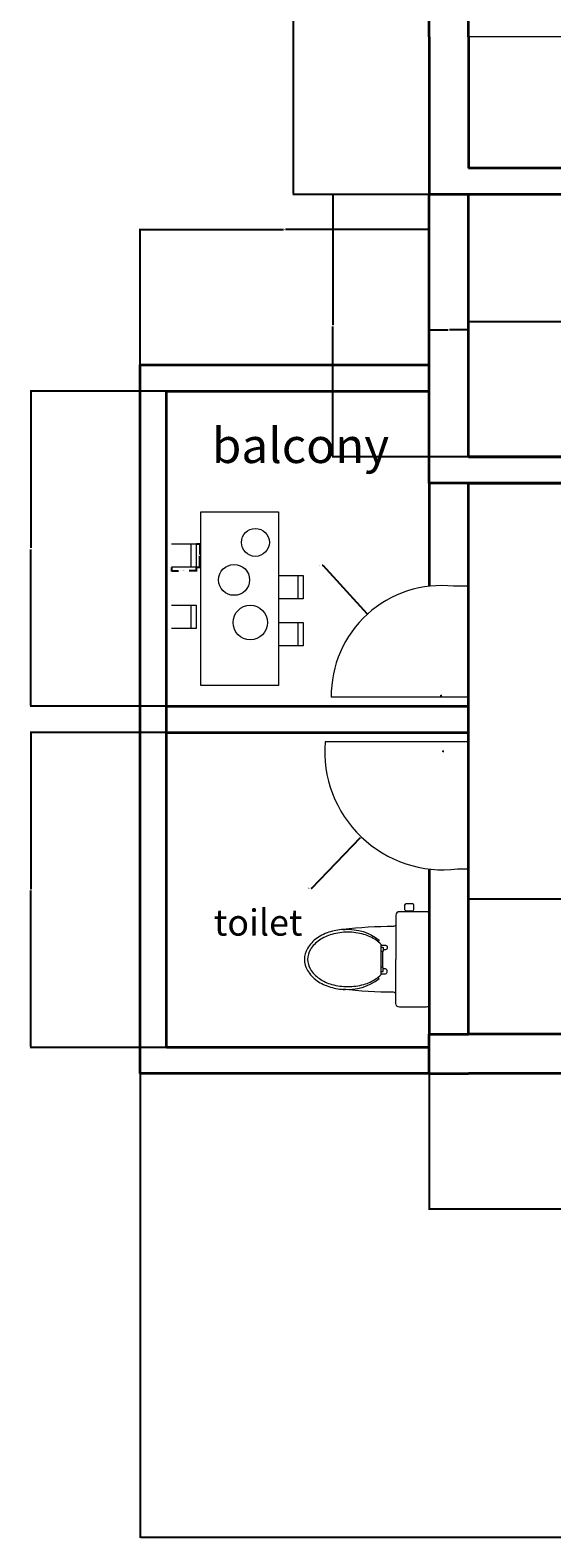
# Model space of a CAD drawing. Units: inches. Extents: x 177 to 785, y -381 to 206.
# Tile 1 of 5: x 177 to 296, y -381 to -37. Entities that reach past the tile are written whole.
import ezdxf

# ---------------------------------------------------------------- set-up
doc = ezdxf.new("R2010")
doc.units = ezdxf.units.IN
doc.header["$MEASUREMENT"] = 0
for name, color, linetype, lineweight in [('A-ANNO-DIMS', 2, 'Continuous', 18), ('A-AREA-IDEN', 7, 'Continuous', 20), ('A-DOOR', 4, 'Continuous', 18), ('A-FLOR-FIXT', 8, 'Continuous', 18), ('A-FURN', 2, 'Continuous', 18), ('A-WALL', 7, 'Continuous', 35), ('WC-Detail_dwgmodels.com', 9, 'Continuous', 13), ('WC-Outline_dwgmodels.com', 8, 'Continuous', 18)]:
    doc.layers.add(name, color=color, linetype=linetype, lineweight=lineweight)
doc.styles.get("Standard").update_dxf_attribs({"font": 'arial.ttf'})
doc.dimstyles.get("Standard").update_dxf_attribs({"dimtxt": 0.18, "dimasz": 0.18, "dimexe": 0.18, "dimexo": 0.0625, "dimgap": 0.09, "dimtad": 0, "dimtih": 1, "dimtoh": 1, "dimdec": 4, "dimzin": 0, "dimdsep": 46, "dimtxsty": 'Standard', "dimcen": 0.09, "dimadec": 0, "dimazin": 0, "dimtfac": 1, "dimtdec": 4, "dimtofl": 0, "dimtmove": 0, "dimatfit": 3, "dimfxl": 1, "dimtolj": 1, "dimtzin": 0, "dimarcsym": 0})

# ---------------------------------------------------------------- blocks, each defined once
blk = doc.blocks.new('BED-DOUBLE')
blk.add_line((58.96, 86.04), (58.96, 0))
for points in [[(0, 86.04), (102.05, 86.04), (102.05, 0), (0, 0)], [(70.1, 73.56), (83.84, 73.56), (83.84, 43.2), (70.1, 43.2)], [(70.1, 37.79), (83.84, 37.79), (83.84, 7.42), (70.1, 7.42)]]:
    blk.add_lwpolyline(points, close=True)
blk = doc.blocks.new('CHAIR-BALCONY-SMALL')
for p, q in [((0, 5.34), (4.46, 5.34)), ((4.46, 5.34), (4.46, 0)), ((4.46, 5.34), (5.66, 5.34)), ((5.66, 5.34), (5.66, 0)), ((4.46, 0), (0, 0)), ((5.66, 0), (4.46, 0))]:
    blk.add_line(p, q)
blk = doc.blocks.new('WC-PAN-AND-SEAT')
for points in [[(0, 20.91, -0.279901), (0.43, 20.4, 0.030761), (1.12, 8.8, 16.522544)], [(15.88, 20.91, 0.279901), (15.45, 20.4, -0.030761), (14.76, 8.8, -16.522544)], [(1.72, 9.92, 0.068564), (2.22, 6.28, 0.080689), (3.54, 3.43, 0.107047), (5.7, 1.38, 0.137952), (7.94, 0.75, 0.137952), (10.18, 1.38, 0.107047), (12.34, 3.43, 0.080689), (13.66, 6.28, 0.068564), (14.16, 9.92, 0.068564), (13.66, 13.57, 0.080689), (12.34, 16.41, 0.049741), (11.45, 17.48, 0.137952)], [(4.44, 17.48, 0.049741), (3.54, 16.41, 0.080689), (2.22, 13.57, 0.068564), (1.72, 9.92, 0.068564)], [(1.08, 9.29, -0.186192), (3.55, 17.08), (3.86, 16.84)], [(14.76, 8.8, 0.197511), (12.33, 17.08), (12.02, 16.84)], [(1.07, 9.29, 0.059006), (1.61, 5.99, 0.081908), (3.07, 2.91, 0.106902), (5.45, 0.69, 0.135271), (7.94, 0, 0.135271)], [(1.12, 8.8, -0.010918), (1.08, 9.29)], [(7.94, 0, 0.135271), (10.44, 0.69, 0.106902), (12.81, 2.91, 0.081908), (14.28, 5.99, 0.059006), (14.82, 9.29, 0.070136)]]:
    blk.add_lwpolyline(points, format="xyb")
blk.add_lwpolyline([(4.44, 17.48), (11.45, 17.48)])
blk = doc.blocks.new('*D11')
at = {"layer": 'A-ANNO-DIMS', "color": 0, "lineweight": -2, "transparency": 16777216}
for p, q in [((209.45, -159.41), (209.45, -160.37)), ((209.63, -160.19), (211.07, -160.19)), ((214.93, -160.19), (213.49, -160.19)), ((215.11, -159.41), (215.11, -160.37))]:
    blk.add_line(p, q, dxfattribs=at)
at = {"layer": 'A-ANNO-DIMS', "color": 0, "transparency": 16777216}
for points in [[(209.63, -160.16), (209.63, -160.22), (209.45, -160.19)], [(214.93, -160.16), (214.93, -160.22), (215.11, -160.19)]]:
    blk.add_solid(points, dxfattribs=at)
at = {"layer": 'Defpoints', "color": 0, "transparency": 16777216}
for p in [(209.45, -159.35), (215.11, -159.35), (215.11, -160.19)]:
    blk.add_point(p, dxfattribs=at)
at = {"layer": 'A-ANNO-DIMS', "color": 0, "transparency": 16777216, "insert": (212.28, -160.19), "char_height": 0.18, "attachment_point": 5}
blk.add_mtext('\\A1;SIDE CHAIR 6 TYP.', dxfattribs=at)
blk = doc.blocks.new('*D12')
at = {"layer": 'A-ANNO-DIMS', "color": 0, "lineweight": -2, "transparency": 16777216}
for p, q in [((215.18, -154.01), (216.14, -154.01)), ((215.96, -154.19), (215.96, -156.5)), ((215.96, -159.17), (215.96, -156.86)), ((215.18, -159.35), (216.14, -159.35))]:
    blk.add_line(p, q, dxfattribs=at)
at = {"layer": 'A-ANNO-DIMS', "color": 0, "transparency": 16777216}
for points in [[(215.93, -154.19), (215.99, -154.19), (215.96, -154.01)], [(215.93, -159.17), (215.99, -159.17), (215.96, -159.35)]]:
    blk.add_solid(points, dxfattribs=at)
at = {"layer": 'Defpoints', "color": 0, "transparency": 16777216}
for p in [(215.11, -154.01), (215.96, -154.01), (215.11, -159.35)]:
    blk.add_point(p, dxfattribs=at)
at = {"layer": 'A-ANNO-DIMS', "color": 0, "transparency": 16777216, "insert": (215.96, -156.68), "char_height": 0.18, "attachment_point": 5}
blk.add_mtext('\\A1;5 TYP.', dxfattribs=at)
blk = doc.blocks.new('*D23')
at = {"layer": 'A-ANNO-DIMS', "color": 0, "lineweight": -2, "transparency": 16777216}
for p, q in [((754.33, -257.2), (754.33, -381.27)), ((202.33, -275.2), (202.33, -381.27)), ((202.51, -381.09), (478.04, -381.09)), ((754.15, -381.09), (478.62, -381.09))]:
    blk.add_line(p, q, dxfattribs=at)
at = {"layer": 'A-ANNO-DIMS', "color": 0, "transparency": 16777216}
for points in [[(202.51, -381.06), (202.51, -381.12), (202.33, -381.09)], [(754.15, -381.06), (754.15, -381.12), (754.33, -381.09)]]:
    blk.add_solid(points, dxfattribs=at)
at = {"layer": 'Defpoints', "color": 0, "transparency": 16777216}
for p in [(754.33, -257.14), (202.33, -275.14), (754.33, -381.09)]:
    blk.add_point(p, dxfattribs=at)
at = {"layer": 'A-ANNO-DIMS', "color": 0, "transparency": 16777216, "insert": (478.33, -381.09), "char_height": 0.18, "attachment_point": 5}
blk.add_mtext('\\A1;552', dxfattribs=at)
blk = doc.blocks.new('*D25')
at = {"layer": 'A-ANNO-DIMS', "color": 0, "lineweight": -2, "transparency": 16777216}
for p, q in [((202.33, -113.08), (202.33, -82.01)), ((202.51, -82.19), (235.11, -82.19)), ((268.15, -82.19), (235.55, -82.19)), ((268.33, -113.08), (268.33, -82.01))]:
    blk.add_line(p, q, dxfattribs=at)
at = {"layer": 'A-ANNO-DIMS', "color": 0, "transparency": 16777216}
for points in [[(202.51, -82.16), (202.51, -82.22), (202.33, -82.19)], [(268.15, -82.16), (268.15, -82.22), (268.33, -82.19)]]:
    blk.add_solid(points, dxfattribs=at)
at = {"layer": 'Defpoints', "color": 0, "transparency": 16777216}
for p in [(268.33, -82.19), (202.33, -113.14), (268.33, -113.14)]:
    blk.add_point(p, dxfattribs=at)
at = {"layer": 'A-ANNO-DIMS', "color": 0, "transparency": 16777216, "insert": (235.33, -82.19), "char_height": 0.18, "attachment_point": 5}
blk.add_mtext('\\A1;66', dxfattribs=at)
blk = doc.blocks.new('*D37')
at = {"layer": 'A-ANNO-DIMS', "color": 0, "lineweight": -2, "transparency": 16777216}
for p, q in [((268.27, 102.86), (237.2, 102.86)), ((237.38, 102.68), (237.38, 14.54)), ((237.38, -73.96), (237.38, 14.18)), ((268.27, -74.14), (237.2, -74.14))]:
    blk.add_line(p, q, dxfattribs=at)
at = {"layer": 'A-ANNO-DIMS', "color": 0, "transparency": 16777216}
for points in [[(237.35, 102.68), (237.41, 102.68), (237.38, 102.86)], [(237.35, -73.96), (237.41, -73.96), (237.38, -74.14)]]:
    blk.add_solid(points, dxfattribs=at)
at = {"layer": 'Defpoints', "color": 0, "transparency": 16777216}
for p in [(237.38, 102.86), (268.33, 102.86), (268.33, -74.14)]:
    blk.add_point(p, dxfattribs=at)
at = {"layer": 'A-ANNO-DIMS', "color": 0, "transparency": 16777216, "insert": (237.38, 14.36), "char_height": 0.18, "attachment_point": 5}
blk.add_mtext('\\A1;177', dxfattribs=at)
blk = doc.blocks.new('*D41')
at = {"layer": 'A-ANNO-DIMS', "color": 0, "lineweight": -2, "transparency": 16777216}
for p, q in [((277.33, -134.08), (277.33, -103.01)), ((277.51, -103.19), (321.11, -103.19)), ((365.15, -103.19), (321.55, -103.19)), ((365.33, -134.08), (365.33, -103.01))]:
    blk.add_line(p, q, dxfattribs=at)
at = {"layer": 'A-ANNO-DIMS', "color": 0, "transparency": 16777216}
for points in [[(277.51, -103.16), (277.51, -103.22), (277.33, -103.19)], [(365.15, -103.16), (365.15, -103.22), (365.33, -103.19)]]:
    blk.add_solid(points, dxfattribs=at)
at = {"layer": 'Defpoints', "color": 0, "transparency": 16777216}
for p in [(365.33, -103.19), (277.33, -134.14), (365.33, -134.14)]:
    blk.add_point(p, dxfattribs=at)
at = {"layer": 'A-ANNO-DIMS', "color": 0, "transparency": 16777216, "insert": (321.33, -103.19), "char_height": 0.18, "attachment_point": 5}
blk.add_mtext('\\A1;88', dxfattribs=at)
blk = doc.blocks.new('*D42')
at = {"layer": 'A-ANNO-DIMS', "color": 0, "lineweight": -2, "transparency": 16777216}
for p, q in [((277.27, -74.14), (246.2, -74.14)), ((246.38, -74.32), (246.38, -103.96)), ((246.38, -133.96), (246.38, -104.32)), ((277.27, -134.14), (246.2, -134.14))]:
    blk.add_line(p, q, dxfattribs=at)
at = {"layer": 'A-ANNO-DIMS', "color": 0, "transparency": 16777216}
for points in [[(246.35, -74.32), (246.41, -74.32), (246.38, -74.14)], [(246.35, -133.96), (246.41, -133.96), (246.38, -134.14)]]:
    blk.add_solid(points, dxfattribs=at)
at = {"layer": 'Defpoints', "color": 0, "transparency": 16777216}
for p in [(246.38, -74.14), (277.33, -74.14), (277.33, -134.14)]:
    blk.add_point(p, dxfattribs=at)
at = {"layer": 'A-ANNO-DIMS', "color": 0, "transparency": 16777216, "insert": (246.38, -104.14), "char_height": 0.18, "attachment_point": 5}
blk.add_mtext('\\A1;60', dxfattribs=at)
blk = doc.blocks.new('*D43')
at = {"layer": 'A-ANNO-DIMS', "color": 0, "lineweight": -2, "transparency": 16777216}
for p, q in [((208.27, -119.14), (177.2, -119.14)), ((177.38, -119.32), (177.38, -154.96)), ((177.38, -190.96), (177.38, -155.32)), ((208.27, -191.14), (177.2, -191.14))]:
    blk.add_line(p, q, dxfattribs=at)
at = {"layer": 'A-ANNO-DIMS', "color": 0, "transparency": 16777216}
for points in [[(177.35, -119.32), (177.41, -119.32), (177.38, -119.14)], [(177.35, -190.96), (177.41, -190.96), (177.38, -191.14)]]:
    blk.add_solid(points, dxfattribs=at)
at = {"layer": 'Defpoints', "color": 0, "transparency": 16777216}
for p in [(177.38, -119.14), (208.33, -119.14), (208.33, -191.14)]:
    blk.add_point(p, dxfattribs=at)
at = {"layer": 'A-ANNO-DIMS', "color": 0, "transparency": 16777216, "insert": (177.38, -155.14), "char_height": 0.18, "attachment_point": 5}
blk.add_mtext('\\A1;72', dxfattribs=at)
blk = doc.blocks.new('*D44')
at = {"layer": 'A-ANNO-DIMS', "color": 0, "lineweight": -2, "transparency": 16777216}
for p, q in [((208.27, -197.14), (177.2, -197.14)), ((177.38, -197.32), (177.38, -232.96)), ((177.38, -268.96), (177.38, -233.32)), ((208.27, -269.14), (177.2, -269.14))]:
    blk.add_line(p, q, dxfattribs=at)
at = {"layer": 'A-ANNO-DIMS', "color": 0, "transparency": 16777216}
for points in [[(177.35, -197.32), (177.41, -197.32), (177.38, -197.14)], [(177.35, -268.96), (177.41, -268.96), (177.38, -269.14)]]:
    blk.add_solid(points, dxfattribs=at)
at = {"layer": 'Defpoints', "color": 0, "transparency": 16777216}
for p in [(177.38, -197.14), (208.33, -197.14), (208.33, -269.14)]:
    blk.add_point(p, dxfattribs=at)
at = {"layer": 'A-ANNO-DIMS', "color": 0, "transparency": 16777216, "insert": (177.38, -233.14), "char_height": 0.18, "attachment_point": 5}
blk.add_mtext('\\A1;72', dxfattribs=at)
blk = doc.blocks.new('*D45')
at = {"layer": 'A-ANNO-DIMS', "color": 0, "lineweight": -2, "transparency": 16777216}
for p, q in [((277.33, -266.08), (277.33, -235.01)), ((277.51, -235.19), (370.05, -235.19)), ((463.15, -235.19), (370.61, -235.19)), ((463.33, -266.08), (463.33, -235.01))]:
    blk.add_line(p, q, dxfattribs=at)
at = {"layer": 'A-ANNO-DIMS', "color": 0, "transparency": 16777216}
for points in [[(277.51, -235.16), (277.51, -235.22), (277.33, -235.19)], [(463.15, -235.16), (463.15, -235.22), (463.33, -235.19)]]:
    blk.add_solid(points, dxfattribs=at)
at = {"layer": 'Defpoints', "color": 0, "transparency": 16777216}
for p in [(463.33, -235.19), (277.33, -266.14), (463.33, -266.14)]:
    blk.add_point(p, dxfattribs=at)
at = {"layer": 'A-ANNO-DIMS', "color": 0, "transparency": 16777216, "insert": (370.33, -235.19), "char_height": 0.18, "attachment_point": 5}
blk.add_mtext('\\A1;186', dxfattribs=at)
blk = doc.blocks.new('*D63')
at = {"layer": 'A-ANNO-DIMS', "color": 0, "lineweight": -2, "transparency": 16777216}
for p, q in [((268.33, -74.2), (268.33, -105.27)), ((277.33, -74.2), (277.33, -105.27)), ((268.51, -105.09), (272.68, -105.09)), ((277.15, -105.09), (272.98, -105.09))]:
    blk.add_line(p, q, dxfattribs=at)
at = {"layer": 'A-ANNO-DIMS', "color": 0, "transparency": 16777216}
for points in [[(268.51, -105.06), (268.51, -105.12), (268.33, -105.09)], [(277.15, -105.06), (277.15, -105.12), (277.33, -105.09)]]:
    blk.add_solid(points, dxfattribs=at)
at = {"layer": 'Defpoints', "color": 0, "transparency": 16777216}
for p in [(268.33, -74.14), (277.33, -74.14), (268.33, -105.09)]:
    blk.add_point(p, dxfattribs=at)
at = {"layer": 'A-ANNO-DIMS', "color": 0, "transparency": 16777216, "insert": (272.83, -105.09), "char_height": 0.18, "attachment_point": 5}
blk.add_mtext('\\A1;9', dxfattribs=at)
blk = doc.blocks.new('*D65')
at = {"layer": 'A-ANNO-DIMS', "color": 0, "lineweight": -2, "transparency": 16777216}
for p, q in [((268.33, -275.2), (268.33, -306.27)), ((362.7, -275.2), (362.7, -306.27)), ((268.51, -306.09), (315.12, -306.09)), ((362.52, -306.09), (315.91, -306.09))]:
    blk.add_line(p, q, dxfattribs=at)
at = {"layer": 'A-ANNO-DIMS', "color": 0, "transparency": 16777216}
for points in [[(268.51, -306.06), (268.51, -306.12), (268.33, -306.09)], [(362.52, -306.06), (362.52, -306.12), (362.7, -306.09)]]:
    blk.add_solid(points, dxfattribs=at)
at = {"layer": 'Defpoints', "color": 0, "transparency": 16777216}
for p in [(268.33, -275.14), (362.7, -275.14), (268.33, -306.09)]:
    blk.add_point(p, dxfattribs=at)
at = {"layer": 'A-ANNO-DIMS', "color": 0, "transparency": 16777216, "insert": (315.51, -306.09), "char_height": 0.18, "attachment_point": 5}
blk.add_mtext('\\A1;94.37', dxfattribs=at)
blk = doc.blocks.new('*D81')
at = {"layer": 'A-ANNO-DIMS', "color": 0, "lineweight": -2, "transparency": 16777216}
for p, q in [((271.49, -201.46), (271.67, -201.46)), ((271.58, -201.55), (271.58, -201.37)), ((241.55, -232.74), (252.69, -221.14)), ((241.37, -232.74), (241.55, -232.74))]:
    blk.add_line(p, q, dxfattribs=at)
at = {"layer": 'A-ANNO-DIMS', "color": 0, "transparency": 16777216}
blk.add_solid([(252.67, -221.12), (252.71, -221.16), (252.81, -221.01)], dxfattribs=at)
at = {"layer": 'Defpoints', "color": 0, "transparency": 16777216}
for p in [(271.58, -201.46), (252.81, -221.01)]:
    blk.add_point(p, dxfattribs=at)
at = {"layer": 'A-ANNO-DIMS', "color": 0, "transparency": 16777216, "insert": (240.98, -232.74), "char_height": 0.18, "attachment_point": 5}
blk.add_mtext('\\A1;R27.1', dxfattribs=at)
blk = doc.blocks.new('*D82')
at = {"layer": 'A-ANNO-DIMS', "color": 0, "lineweight": -2, "transparency": 16777216}
for p, q in [((243.91, -158.94), (244.09, -158.94)), ((244.09, -158.94), (254.11, -169.98)), ((271.04, -188.74), (271.22, -188.74)), ((271.13, -188.83), (271.13, -188.65))]:
    blk.add_line(p, q, dxfattribs=at)
at = {"layer": 'A-ANNO-DIMS', "color": 0, "transparency": 16777216}
blk.add_solid([(254.13, -169.96), (254.09, -170), (254.23, -170.12)], dxfattribs=at)
at = {"layer": 'Defpoints', "color": 0, "transparency": 16777216}
for p in [(254.23, -170.12), (271.13, -188.74)]:
    blk.add_point(p, dxfattribs=at)
at = {"layer": 'A-ANNO-DIMS', "color": 0, "transparency": 16777216, "insert": (243.36, -158.94), "char_height": 0.18, "attachment_point": 5}
blk.add_mtext('\\A1;R25.154', dxfattribs=at)

msp = doc.modelspace()

# ---------------------------------------------------------------- linework, layer by layer
at = {"layer": 'A-DOOR'}
for p, q in [((277.3284, -163.747), (273.9385, -163.747)), ((277.3284, -189.1135), (245.9824, -189.1135)), ((277.3284, -199.3112), (244.5649, -199.3112)), ((274.831, -228.3623), (277.3284, -228.3623))]:
    msp.add_line(p, q, dxfattribs=at)
for centre, radius, start, end in [((271.1335, -188.7439), 25.1538, 83.597313, 180.841855), ((271.5797, -201.4581), 27.0999, 175.456331, 276.89064)]:
    msp.add_arc(centre, radius, start, end, dxfattribs=at)
at = {"layer": 'A-FURN'}
msp.add_lwpolyline([(233.922, -146.7244), (233.922, -186.455), (216.2174, -186.455), (216.2174, -146.7244)], close=True, dxfattribs=at)
for centre, radius in [((228.6587, -153.7125), 3.1895), ((223.7905, -162.2801), 3.5279), ((227.4836, -172.0238), 3.9345)]:
    msp.add_circle(centre, radius, dxfattribs=at)
at = {"layer": 'A-WALL'}
for p, q in [((268.3284, -38.1401), (268.3284, 93.8599)), ((277.3284, -38.1401), (277.3284, 93.8599)), ((268.3284, -38.1401), (268.3284, -74.1401)), ((277.3284, -38.1401), (277.3284, -68.1401)), ((371.3284, -68.1401), (277.3284, -68.1401)), ((277.3284, -74.1401), (268.3284, -74.1401)), ((268.3284, -134.1401), (268.3284, -74.1401)), ((277.3284, -134.1401), (277.3284, -74.1401)), ((365.3284, -74.1401), (277.3284, -74.1401)), ((202.3284, -119.1401), (202.3284, -113.1401)), ((202.3284, -113.1401), (208.3284, -113.1401)), ((208.3284, -113.1401), (268.3284, -113.1401)), ((202.3284, -191.1401), (202.3284, -119.1401)), ((208.3284, -191.1401), (208.3284, -119.1401)), ((208.3284, -119.1401), (268.3284, -119.1401)), ((268.3284, -140.1401), (268.3284, -134.1401)), ((365.3284, -134.1401), (277.3284, -134.1401)), ((277.3284, -134.1401), (365.3284, -134.1401)), ((277.3284, -140.1401), (268.3284, -140.1401)), ((268.3284, -140.1401), (268.3284, -163.747)), ((365.3284, -140.1401), (277.3284, -140.1401)), ((277.3284, -266.1401), (277.3284, -140.1401)), ((277.3284, -140.1401), (371.3284, -140.1401)), ((202.3284, -275.1401), (202.3284, -191.1401)), ((208.3284, -269.1401), (208.3284, -191.1401)), ((208.3284, -191.1401), (268.3284, -191.1401)), ((268.3284, -191.1401), (277.3284, -191.1401)), ((208.3284, -197.1401), (268.3284, -197.1401)), ((268.3284, -197.1401), (277.3284, -197.1401)), ((268.3284, -228.3623), (268.3284, -266.1401)), ((268.3284, -266.1401), (277.3284, -266.1401)), ((268.3284, -275.1401), (268.3284, -266.1401)), ((433.3284, -266.1401), (277.3284, -266.1401)), ((268.3284, -269.1401), (208.3284, -269.1401)), ((208.3284, -275.1401), (202.3284, -275.1401)), ((268.3284, -275.1401), (208.3284, -275.1401)), ((268.3284, -275.1401), (277.3284, -275.1401)), ((433.3284, -275.1401), (277.3284, -275.1401))]:
    msp.add_line(p, q, dxfattribs=at)
at = {"layer": 'WC-Detail_dwgmodels.com'}
for points in [[(263.1874, -237.8962), (264.4472, -237.8962, 0.41421356)], [(257.3212, -245.7702), (258.3448, -245.7702, -0.78819772), (258.3448, -246.8726), (257.8724, -246.8726)], [(257.3212, -246.2427), (257.6755, -246.2427, -0.41421356), (257.8724, -246.4395), (257.8724, -247.0301, -0.41421356), (257.6755, -247.2269), (257.3212, -247.2269)], [(257.3212, -251.8332), (257.6755, -251.8332, 0.41421356), (257.8724, -251.6364), (257.8724, -251.0458, 0.41421356), (257.6755, -250.849), (257.3212, -250.849)], [(257.3212, -252.3057), (258.3448, -252.3057, 0.78819772), (258.3448, -251.2033), (257.8724, -251.2033)]]:
    msp.add_lwpolyline(points, format="xyb", dxfattribs=at)
msp.add_lwpolyline([(257.7149, -247.2269), (257.7149, -250.849)], dxfattribs=at)
at = {"layer": 'WC-Outline_dwgmodels.com'}
for points in [[(264.4472, -237.8962), (264.6047, -237.8962, 0.41421356), (264.8803, -237.6206), (264.8803, -236.6364, 0.41421356), (264.6047, -236.3608), (263.0299, -236.3608, 0.41421356), (262.7543, -236.6364)], [(262.7543, -236.6364), (262.7543, -237.6206, 0.41421356), (263.0299, -237.8962), (263.1874, -237.8962, 0.41421356)], [(263.1874, -238.1324), (261.5732, -238.1324, 0.41421356), (260.7464, -238.9592), (260.7464, -241.0963)], [(264.4472, -238.1324), (263.1874, -238.1324, 0.41421356)], [(268.5417, -249.038), (268.5417, -238.9592, 0.41421356), (267.7149, -238.1324), (264.4472, -238.1324, 0.41421356)], [(268.5417, -249.038), (268.5417, -259.1167, -0.41421356), (267.7149, -259.9435), (261.5732, -259.9435, -0.41421356), (260.7464, -259.1167), (260.7464, -256.9797)]]:
    msp.add_lwpolyline(points, format="xyb", dxfattribs=at)
for points in [[(260.7464, -241.0963), (260.7464, -249.038)], [(263.1874, -237.8962), (263.1874, -238.1324)], [(264.4472, -237.8962), (264.4472, -238.1324)], [(260.7464, -256.9797), (260.7464, -249.038)]]:
    msp.add_lwpolyline(points, dxfattribs=at)

# ---------------------------------------------------------------- block references
at = {"layer": 'A-FLOR-FIXT', "rotation": 270.0000000000001}
msp.add_blockref('WC-PAN-AND-SEAT', (239.841, -241.0963), dxfattribs=at)
at = {"layer": 'A-FURN', "rotation": 180}
msp.add_blockref('BED-DOUBLE', (379.3818, 47.9038), dxfattribs=at)
at = {"layer": 'A-FURN'}
for p in [(209.4517, -159.3457), (233.922, -166.59), (209.4517, -173.4234), (233.922, -177.3245)]:
    msp.add_blockref('CHAIR-BALCONY-SMALL', p, dxfattribs=at)

# ---------------------------------------------------------------- texts
at = {"layer": 'A-AREA-IDEN', "attachment_point": 1}
for s, heights, insert, char_height in [('balcony', [6.0982], (218.6975, -127.5601), 8), ('toilet', [0], (219.1563, -237.6058), 6)]:
    msp.add_mtext_dynamic_manual_height_columns(s, width=20.406791, gutter_width=1, heights=heights, dxfattribs=dict(at, insert=insert, char_height=char_height))

# ---------------------------------------------------------------- dimensions: what is measured, and where the dimension line sits
at = {"layer": 'A-ANNO-DIMS'}
for base, p1, p2, angle, override, picture, middle in [((237.3784, 102.8599), (268.3284, -74.1401), (268.3284, 102.8599), 90, {"dimdec": 0, "dimlfac": 1, "dimrnd": 0, "dimzin": 0, "dimdsep": 46, "dimlunit": 2}, '*D37', (237.3784, 14.3599)), ((246.3784, -74.1401), (277.3284, -134.1401), (277.3284, -74.1401), 90, {"dimdec": 0, "dimlfac": 1, "dimrnd": 0, "dimzin": 0, "dimdsep": 46, "dimlunit": 2}, '*D42', (246.3784, -104.1401)), ((268.3284, -105.0901), (277.3284, -74.1401), (268.3284, -74.1401), 180, {"dimdec": 0, "dimlfac": 1, "dimrnd": 0, "dimzin": 0, "dimdsep": 46, "dimlunit": 2}, '*D63', (272.8284, -105.0901)), ((177.3784, -119.1401), (208.3284, -191.1401), (208.3284, -119.1401), 90, {"dimdec": 0, "dimlfac": 1, "dimrnd": 0, "dimzin": 0, "dimdsep": 46, "dimlunit": 2}, '*D43', (177.3784, -155.1401)), ((177.3784, -197.1401), (208.3284, -269.1401), (208.3284, -197.1401), 90, {"dimdec": 0, "dimlfac": 1, "dimrnd": 0, "dimzin": 0, "dimdsep": 46, "dimlunit": 2}, '*D44', (177.3784, -233.1401)), ((268.3284, -306.0901), (362.6997, -275.1401), (268.3284, -275.1401), 180, {"dimdec": 2, "dimlfac": 1, "dimrnd": 0, "dimzin": 0, "dimdsep": 46, "dimlunit": 2}, '*D65', (315.5141, -306.0901))]:
    dim = msp.add_linear_dim(base=base, p1=p1, p2=p2, angle=angle, dimstyle='Standard', override=override, dxfattribs=at)
    dim.commit()
    dim.dimension.update_dxf_attribs({"geometry": picture, "text_midpoint": middle})
for base, p1, p2, picture, middle in [((268.3284, -82.1901), (202.3284, -113.1401), (268.3284, -113.1401), '*D25', (235.3284, -82.1901)), ((365.3284, -103.1901), (277.3284, -134.1401), (365.3284, -134.1401), '*D41', (321.3284, -103.1901)), ((463.3284, -235.1901), (277.3284, -266.1401), (463.3284, -266.1401), '*D45', (370.3284, -235.1901)), ((754.3284, -381.0901), (202.3284, -275.1401), (754.3284, -257.1401), '*D23', (478.3284, -381.0901))]:
    dim = msp.add_linear_dim(base=base, p1=p1, p2=p2, dimstyle='Standard', override={"dimdec": 0, "dimlfac": 1, "dimrnd": 0, "dimzin": 0, "dimdsep": 46, "dimlunit": 2}, dxfattribs=at)
    dim.commit()
    dim.dimension.update_dxf_attribs({"geometry": picture, "text_midpoint": middle})
dim = msp.add_linear_dim(base=(215.963, -154.0101), p1=(215.1137, -159.3454), p2=(215.1137, -154.0101), angle=90, text='<> TYP.', dimstyle='Standard', override={"dimdec": 0, "dimlfac": 1, "dimrnd": 0, "dimzin": 0, "dimdsep": 46, "dimlunit": 2}, dxfattribs=at)
dim.commit()
dim.dimension.update_dxf_attribs({"geometry": '*D12', "text_midpoint": (215.963, -156.6777)})
dim = msp.add_linear_dim(base=(215.1137, -160.1947), p1=(209.4517, -159.3454), p2=(215.1137, -159.3454), text='SIDE CHAIR <> TYP.', dimstyle='Standard', override={"dimdec": 0, "dimlfac": 1, "dimrnd": 0, "dimzin": 0, "dimdsep": 46, "dimlunit": 2}, dxfattribs=at)
dim.commit()
dim.dimension.update_dxf_attribs({"geometry": '*D11', "text_midpoint": (212.2827, -160.1947)})
for center, mpoint, override, picture, middle in [((271.1335, -188.7439), (254.2307, -170.1157), {"dimdec": 3, "dimlfac": 1, "dimrnd": 0, "dimzin": 0, "dimdsep": 46, "dimlunit": 2}, '*D82', (243.3596, -158.9387)), ((271.5797, -201.4581), (252.8138, -221.0092), {"dimdec": 1, "dimlfac": 1, "dimrnd": 0, "dimzin": 0, "dimdsep": 46, "dimlunit": 2}, '*D81', (240.9817, -232.7399))]:
    dim = msp.add_radius_dim(center=center, mpoint=mpoint, dimstyle='Standard', override=override, dxfattribs=at)
    dim.commit()
    dim.dimension.update_dxf_attribs({"geometry": picture, "text_midpoint": middle, "dimtype": 164})

doc.saveas('drawing.dxf')
